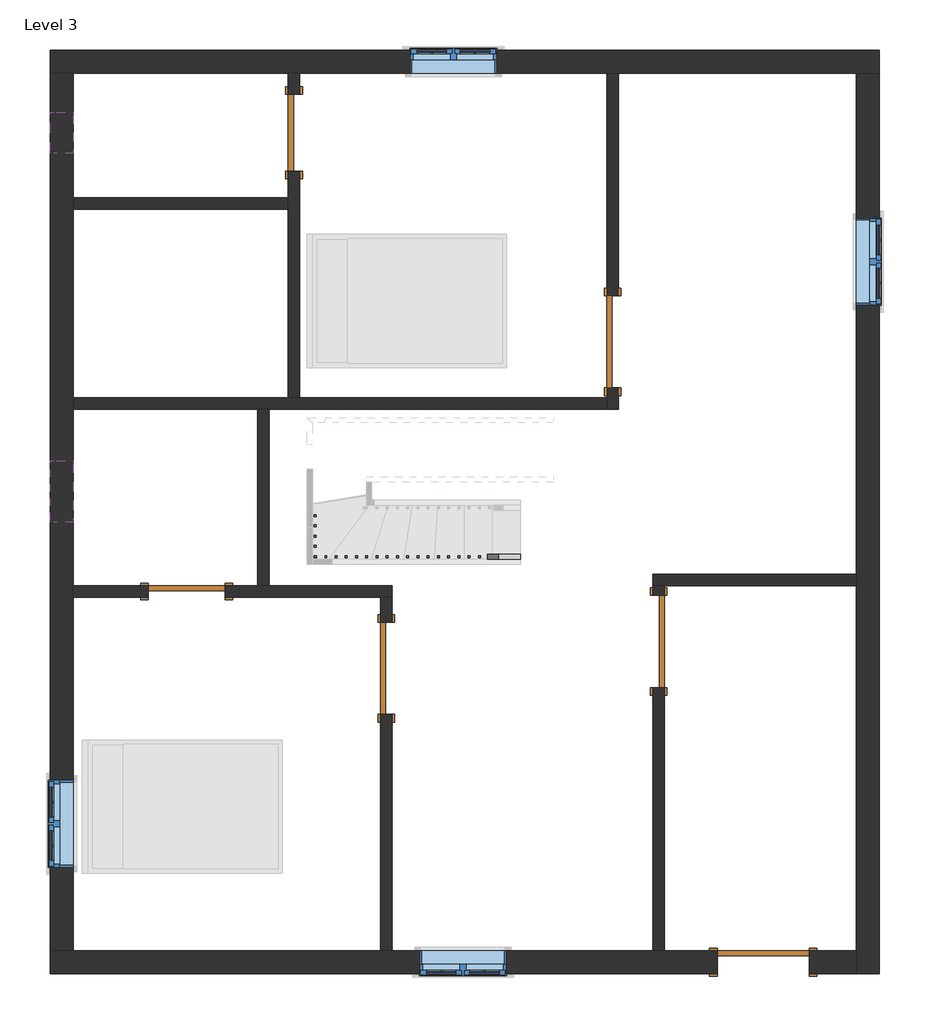
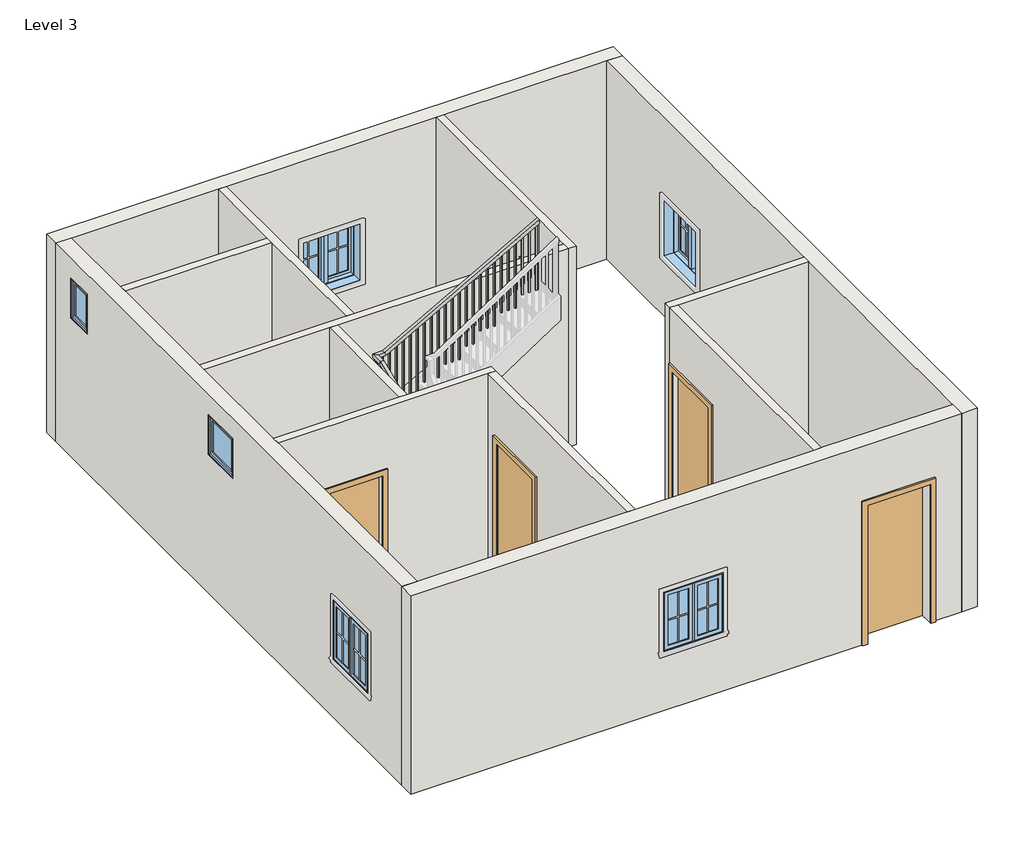
# One storey, part 1 of 2: 13 walls, 6 doors, 6 windows, 1 railing.
"""IFC4 building model written with IfcOpenShell, lengths in millimetres."""

from ifc_helpers import new_model, si_unit, frame, origin, place, context, project, spatial, polyline, outline, extrude, faceted_brep, transform, mapped, element, save
from components import door_d8f5dbb5, door_f2b275c1, door_305aa2a5, door_e5f9f3c4, door_0ca8825f, window_aa618e30, window_80340324, window_339605e1

model = new_model("IFC4")

# Units and contexts
model_context = context("Model", 3, world=origin())
ifc_project = project(units=[si_unit("LENGTHUNIT", "METRE", prefix="MILLI")], contexts=[model_context])

# Site, building, storey
site = spatial("IfcSite", under=ifc_project)
building = spatial("IfcBuilding", under=site)
storey = spatial("IfcBuildingStorey", under=building, Name="Level 3", Elevation=3200.4)

# Doors
placement = place(None, origin())
door_shape = door_d8f5dbb5(model_context)
element("IfcDoor", 1, ObjectType="Single-Flush : 30\" x 80\"", at=placement, inside=storey, context=model_context, shape_type="MappedRepresentation", body=[
    mapped(door_shape, transform((-2510.1648498, 3958.5558073, 3200.4), x_axis=(0.0, 1.0, 0.0), y_axis=(-1.0, 0.0, 0.0), z_axis=(0.0, 0.0, 1.0))),
])
door_2_shape = door_f2b275c1(model_context)
element("IfcDoor", 2, ObjectType="Single-Flush : 30\" x 80\"", at=placement, inside=storey, context=model_context, shape_type="MappedRepresentation", body=[
    mapped(door_2_shape, transform((-3576.9648498, -592.8066927, 3200.4), x_axis=(-1.0, 0.0, 0.0), y_axis=(0.0, -1.0, 0.0), z_axis=(0.0, 0.0, 1.0))),
])
door_3_shape = door_305aa2a5(model_context)
element("IfcDoor", 3, ObjectType="Single-Flush : 36\" x 84\"", at=placement, inside=storey, context=model_context, shape_type="MappedRepresentation", body=[
    mapped(door_3_shape, transform((652.1351502, 1883.6933073, 3200.4), x_axis=(0.0, -1.0, 0.0), y_axis=(1.0, 0.0, 0.0), z_axis=(0.0, 0.0, 1.0))),
])
element("IfcDoor", 4, ObjectType="Single-Flush : 36\" x 84\"", at=placement, inside=storey, context=model_context, shape_type="MappedRepresentation", body=[
    mapped(door_3_shape, transform((1109.3351502, -1088.1066927, 3200.4), x_axis=(0.0, 1.0, 0.0), y_axis=(-1.0, 0.0, 0.0), z_axis=(0.0, 0.0, 1.0))),
])
door_4_shape = door_e5f9f3c4(model_context)
element("IfcDoor", 5, ObjectType="Single-Flush : 36\" x 84\"", at=placement, inside=storey, context=model_context, shape_type="MappedRepresentation", body=[
    mapped(door_4_shape, transform((-1595.7648498, -1354.8066927, 3200.4), x_axis=(0.0, 1.0, 0.0), y_axis=(-1.0, 0.0, 0.0), z_axis=(0.0, 0.0, 1.0))),
])
door_5_shape = door_0ca8825f(model_context)
element("IfcDoor", 6, ObjectType="Single-Flush : 36\" x 84\"", at=placement, inside=storey, context=model_context, shape_type="MappedRepresentation", body=[
    mapped(door_5_shape, transform((2147.5601502, -4269.4566927, 3200.4), x_axis=(1.0, 0.0, 0.0), y_axis=(0.0, 1.0, 0.0), z_axis=(0.0, 0.0, 1.0))),
])

# Railing
element("IfcRailing", 7, ObjectType="Handrail - Rectangular", at=placement, inside=storey, context=model_context, shape_type="SolidModel", body=[
    faceted_brep([(-264.8831579, -271.8029286, 4284.1333333), (-264.8831579, -271.8029286, 4226.5518622), (-264.8831579, -221.0029286, 4226.5518622), (-264.8831579, -221.0029286, 4284.1333333), (-2203.3957557, -271.8029286, 5318.666441), (-2216.1029055, -271.8029286, 5267.866441), (-2216.1029055, -221.0029286, 5267.866441), (-2203.3957557, -221.0029286, 5318.666441), (-2328.8610857, -271.8029286, 5318.666441), (-2328.8610857, -271.8029286, 5267.866441), (-2278.0610857, -221.0029286, 5267.866441), (-2278.0610857, -221.0029286, 5318.666441), (-2328.8610857, -117.3180853, 5318.666441), (-2328.8610857, -107.2249429, 5267.866441), (-2278.0610857, -107.2249429, 5267.866441), (-2278.0610857, -117.3180853, 5318.666441), (-2328.8610857, 889.2076495, 5735.0648193), (-2328.8610857, 899.300792, 5684.2648193), (-2278.0610857, 899.300792, 5684.2648193), (-2278.0610857, 889.2076495, 5735.0648193), (-2328.8610857, 1080.0895433, 5735.0648193), (-2328.8610857, 1080.0895433, 5684.2648193), (-2278.0610857, 1029.2895433, 5684.2648193), (-2278.0610857, 1029.2895433, 5735.0648193), (-2181.3423106, 1080.0895433, 5735.0648193), (-2168.0744201, 1080.0895433, 5684.2648193), (-2168.0744201, 1029.2895433, 5684.2648193), (-2181.3423106, 1029.2895433, 5735.0648193), (63.4034409, 1080.0895433, 6993.4666667), (63.4034409, 1029.2895433, 6993.4666667), (63.4034409, 1029.2895433, 6935.2287027), (63.4034409, 1080.0895433, 6935.2287027)], [[[0, 1, 2, 3]], [[1, 0, 4, 5]], [[2, 1, 5, 6]], [[3, 2, 6, 7]], [[0, 3, 7, 4]], [[5, 4, 8, 9]], [[6, 5, 9, 10]], [[7, 6, 10, 11]], [[4, 7, 11, 8]], [[9, 8, 12, 13]], [[10, 9, 13, 14]], [[11, 10, 14, 15]], [[8, 11, 15, 12]], [[13, 12, 16, 17]], [[14, 13, 17, 18]], [[15, 14, 18, 19]], [[12, 15, 19, 16]], [[17, 16, 20, 21]], [[18, 17, 21, 22]], [[19, 18, 22, 23]], [[16, 19, 23, 20]], [[21, 20, 24, 25]], [[22, 21, 25, 26]], [[23, 22, 26, 27]], [[20, 23, 27, 24]], [[28, 29, 30, 31]], [[25, 24, 28, 31]], [[26, 25, 31, 30]], [[27, 26, 30, 29]], [[24, 27, 29, 28]]]),
    extrude(outline(polyline([(6913.0348603, 23.8139143), (5909.7333333, 23.8139143), (5909.7333333, 42.8639143), (6923.7142681, 42.8639143), (6913.0348603, 23.8139143)])), frame((0.0, 1045.1645433, 0.0), z_axis=(0.0, 1.0, 0.0), x_axis=(0.0, 0.0, 1.0)), (0.0, 0.0, 1.0), 19.05),
    extrude(outline(polyline([(6856.078019, -77.7860857), (5909.7333333, -77.7860857), (5909.7333333, -58.7360857), (6866.7574267, -58.7360857), (6856.078019, -77.7860857)])), frame((0.0, 1045.1645433, 0.0), z_axis=(0.0, 1.0, 0.0), x_axis=(0.0, 0.0, 1.0)), (0.0, 0.0, 1.0), 19.05),
    extrude(outline(polyline([(6799.1211776, -179.3860857), (5909.7333333, -179.3860857), (5909.7333333, -160.3360857), (6809.8005853, -160.3360857), (6799.1211776, -179.3860857)])), frame((0.0, 1045.1645433, 0.0), z_axis=(0.0, 1.0, 0.0), x_axis=(0.0, 0.0, 1.0)), (0.0, 0.0, 1.0), 19.05),
    extrude(outline(polyline([(6742.1643362, -280.9860857), (5740.4, -280.9860857), (5740.4, -261.9360857), (6752.843744, -261.9360857), (6742.1643362, -280.9860857)])), frame((0.0, 1045.1645433, 0.0), z_axis=(0.0, 1.0, 0.0), x_axis=(0.0, 0.0, 1.0)), (0.0, 0.0, 1.0), 19.05),
    extrude(outline(polyline([(6685.2074948, -382.5860857), (5740.4, -382.5860857), (5740.4, -363.5360857), (6695.8869026, -363.5360857), (6685.2074948, -382.5860857)])), frame((0.0, 1045.1645433, 0.0), z_axis=(0.0, 1.0, 0.0), x_axis=(0.0, 0.0, 1.0)), (0.0, 0.0, 1.0), 19.05),
    extrude(outline(polyline([(6628.2506535, -484.1860857), (5740.4, -484.1860857), (5740.4, -465.1360857), (6638.9300612, -465.1360857), (6628.2506535, -484.1860857)])), frame((0.0, 1045.1645433, 0.0), z_axis=(0.0, 1.0, 0.0), x_axis=(0.0, 0.0, 1.0)), (0.0, 0.0, 1.0), 19.05),
    extrude(outline(polyline([(6571.2938121, -585.7860857), (5571.0666667, -585.7860857), (5571.0666667, -566.7360857), (6581.9732198, -566.7360857), (6571.2938121, -585.7860857)])), frame((0.0, 1045.1645433, 0.0), z_axis=(0.0, 1.0, 0.0), x_axis=(0.0, 0.0, 1.0)), (0.0, 0.0, 1.0), 19.05),
    extrude(outline(polyline([(6514.3369707, -687.3860857), (5571.0666667, -687.3860857), (5571.0666667, -668.3360857), (6525.0163785, -668.3360857), (6514.3369707, -687.3860857)])), frame((0.0, 1045.1645433, 0.0), z_axis=(0.0, 1.0, 0.0), x_axis=(0.0, 0.0, 1.0)), (0.0, 0.0, 1.0), 19.05),
    extrude(outline(polyline([(6457.3801293, -788.9860857), (5571.0666667, -788.9860857), (5571.0666667, -769.9360857), (6468.0595371, -769.9360857), (6457.3801293, -788.9860857)])), frame((0.0, 1045.1645433, 0.0), z_axis=(0.0, 1.0, 0.0), x_axis=(0.0, 0.0, 1.0)), (0.0, 0.0, 1.0), 19.05),
    extrude(outline(polyline([(6400.423288, -890.5860857), (5401.7333333, -890.5860857), (5401.7333333, -871.5360857), (6411.1026957, -871.5360857), (6400.423288, -890.5860857)])), frame((0.0, 1045.1645433, 0.0), z_axis=(0.0, 1.0, 0.0), x_axis=(0.0, 0.0, 1.0)), (0.0, 0.0, 1.0), 19.05),
    extrude(outline(polyline([(6343.4664466, -992.1860857), (5401.7333333, -992.1860857), (5401.7333333, -973.1360857), (6354.1458543, -973.1360857), (6343.4664466, -992.1860857)])), frame((0.0, 1045.1645433, 0.0), z_axis=(0.0, 1.0, 0.0), x_axis=(0.0, 0.0, 1.0)), (0.0, 0.0, 1.0), 19.05),
    extrude(outline(polyline([(6286.5096052, -1093.7860857), (5232.4, -1093.7860857), (5232.4, -1074.7360857), (6297.189013, -1074.7360857), (6286.5096052, -1093.7860857)])), frame((0.0, 1045.1645433, 0.0), z_axis=(0.0, 1.0, 0.0), x_axis=(0.0, 0.0, 1.0)), (0.0, 0.0, 1.0), 19.05),
    extrude(outline(polyline([(6229.5527638, -1195.3860857), (5232.4, -1195.3860857), (5232.4, -1176.3360857), (6240.2321716, -1176.3360857), (6229.5527638, -1195.3860857)])), frame((0.0, 1045.1645433, 0.0), z_axis=(0.0, 1.0, 0.0), x_axis=(0.0, 0.0, 1.0)), (0.0, 0.0, 1.0), 19.05),
    extrude(outline(polyline([(6172.5959225, -1296.9860857), (5232.4, -1296.9860857), (5232.4, -1277.9360857), (6183.2753302, -1277.9360857), (6172.5959225, -1296.9860857)])), frame((0.0, 1045.1645433, 0.0), z_axis=(0.0, 1.0, 0.0), x_axis=(0.0, 0.0, 1.0)), (0.0, 0.0, 1.0), 19.05),
    extrude(outline(polyline([(6115.6390811, -1398.5860857), (5063.0666667, -1398.5860857), (5063.0666667, -1379.5360857), (6126.3184889, -1379.5360857), (6115.6390811, -1398.5860857)])), frame((0.0, 1045.1645433, 0.0), z_axis=(0.0, 1.0, 0.0), x_axis=(0.0, 0.0, 1.0)), (0.0, 0.0, 1.0), 19.05),
    extrude(outline(polyline([(6058.6822397, -1500.1860857), (5063.0666667, -1500.1860857), (5063.0666667, -1481.1360857), (6069.3616475, -1481.1360857), (6058.6822397, -1500.1860857)])), frame((0.0, 1045.1645433, 0.0), z_axis=(0.0, 1.0, 0.0), x_axis=(0.0, 0.0, 1.0)), (0.0, 0.0, 1.0), 19.05),
    extrude(outline(polyline([(6001.7253983, -1601.7860857), (5063.0666667, -1601.7860857), (5063.0666667, -1582.7360857), (6012.4048061, -1582.7360857), (6001.7253983, -1601.7860857)])), frame((0.0, 1045.1645433, 0.0), z_axis=(0.0, 1.0, 0.0), x_axis=(0.0, 0.0, 1.0)), (0.0, 0.0, 1.0), 19.05),
    extrude(outline(polyline([(5944.768557, -1703.3860857), (4893.7333333, -1703.3860857), (4893.7333333, -1684.3360857), (5955.4479647, -1684.3360857), (5944.768557, -1703.3860857)])), frame((0.0, 1045.1645433, 0.0), z_axis=(0.0, 1.0, 0.0), x_axis=(0.0, 0.0, 1.0)), (0.0, 0.0, 1.0), 19.05),
    extrude(outline(polyline([(5887.8117156, -1804.9860857), (4893.7333333, -1804.9860857), (4893.7333333, -1785.9360857), (5898.4911234, -1785.9360857), (5887.8117156, -1804.9860857)])), frame((0.0, 1045.1645433, 0.0), z_axis=(0.0, 1.0, 0.0), x_axis=(0.0, 0.0, 1.0)), (0.0, 0.0, 1.0), 19.05),
    extrude(outline(polyline([(5830.8548742, -1906.5860857), (4893.7333333, -1906.5860857), (4893.7333333, -1887.5360857), (5841.534282, -1887.5360857), (5830.8548742, -1906.5860857)])), frame((0.0, 1045.1645433, 0.0), z_axis=(0.0, 1.0, 0.0), x_axis=(0.0, 0.0, 1.0)), (0.0, 0.0, 1.0), 19.05),
    extrude(outline(polyline([(5773.8980329, -2008.1860857), (4893.7333333, -2008.1860857), (4893.7333333, -1989.1360857), (5784.5774406, -1989.1360857), (5773.8980329, -2008.1860857)])), frame((0.0, 1045.1645433, 0.0), z_axis=(0.0, 1.0, 0.0), x_axis=(0.0, 0.0, 1.0)), (0.0, 0.0, 1.0), 19.05),
    extrude(outline(polyline([(5716.9411915, -2109.7860857), (4724.4, -2109.7860857), (4724.4, -2090.7360857), (5727.6205992, -2090.7360857), (5716.9411915, -2109.7860857)])), frame((0.0, 1045.1645433, 0.0), z_axis=(0.0, 1.0, 0.0), x_axis=(0.0, 0.0, 1.0)), (0.0, 0.0, 1.0), 19.05),
    extrude(outline(polyline([(-2211.3860857, 1064.2145433), (-2192.3360857, 1064.2145433), (-2192.3360857, 1045.1645433), (-2211.3860857, 1045.1645433), (-2211.3860857, 1064.2145433)])), frame((0.0, 0.0, 4724.4), z_axis=(0.0, 0.0, 1.0), x_axis=(1.0, 0.0, 0.0)), (0.0, 0.0, 1.0), 959.8648193),
    extrude(outline(polyline([(-2312.9860857, 963.2720714), (-2312.9860857, 982.3220714), (-2293.9360857, 982.3220714), (-2293.9360857, 963.2720714), (-2312.9860857, 963.2720714)])), frame((0.0, 0.0, 4724.4), z_axis=(0.0, 0.0, 1.0), x_axis=(1.0, 0.0, 0.0)), (0.0, 0.0, 1.0), 959.8648193),
    extrude(outline(polyline([(880.7220714, 5676.5788269), (880.7220714, 4724.4), (861.6720714, 4724.4), (861.6720714, 5668.6978669), (880.7220714, 5676.5788269)])), frame((-2312.9860857, 0.0, 0.0), z_axis=(1.0, 0.0, 0.0), x_axis=(0.0, 1.0, 0.0)), (0.0, 0.0, 1.0), 19.05),
    extrude(outline(polyline([(779.1220714, 5634.54704), (779.1220714, 4724.4), (760.0720714, 4724.4), (760.0720714, 5626.6660799), (779.1220714, 5634.54704)])), frame((-2312.9860857, 0.0, 0.0), z_axis=(1.0, 0.0, 0.0), x_axis=(0.0, 1.0, 0.0)), (0.0, 0.0, 1.0), 19.05),
    extrude(outline(polyline([(677.5220714, 5592.515253), (677.5220714, 4724.4), (658.4720714, 4724.4), (658.4720714, 5584.634293), (677.5220714, 5592.515253)])), frame((-2312.9860857, 0.0, 0.0), z_axis=(1.0, 0.0, 0.0), x_axis=(0.0, 1.0, 0.0)), (0.0, 0.0, 1.0), 19.05),
    extrude(outline(polyline([(575.9220714, 5550.4834661), (575.9220714, 4555.0666667), (556.8720714, 4555.0666667), (556.8720714, 5542.602506), (575.9220714, 5550.4834661)])), frame((-2312.9860857, 0.0, 0.0), z_axis=(1.0, 0.0, 0.0), x_axis=(0.0, 1.0, 0.0)), (0.0, 0.0, 1.0), 19.05),
    extrude(outline(polyline([(474.3220714, 5508.4516792), (474.3220714, 4555.0666667), (455.2720714, 4555.0666667), (455.2720714, 5500.5707191), (474.3220714, 5508.4516792)])), frame((-2312.9860857, 0.0, 0.0), z_axis=(1.0, 0.0, 0.0), x_axis=(0.0, 1.0, 0.0)), (0.0, 0.0, 1.0), 19.05),
    extrude(outline(polyline([(372.7220714, 5466.4198922), (372.7220714, 4555.0666667), (353.6720714, 4555.0666667), (353.6720714, 5458.5389322), (372.7220714, 5466.4198922)])), frame((-2312.9860857, 0.0, 0.0), z_axis=(1.0, 0.0, 0.0), x_axis=(0.0, 1.0, 0.0)), (0.0, 0.0, 1.0), 19.05),
    extrude(outline(polyline([(271.1220714, 5424.3881053), (271.1220714, 4555.0666667), (252.0720714, 4555.0666667), (252.0720714, 5416.5071452), (271.1220714, 5424.3881053)])), frame((-2312.9860857, 0.0, 0.0), z_axis=(1.0, 0.0, 0.0), x_axis=(0.0, 1.0, 0.0)), (0.0, 0.0, 1.0), 19.05),
    extrude(outline(polyline([(169.5220714, 5382.3563183), (169.5220714, 4385.7333333), (150.4720714, 4385.7333333), (150.4720714, 5374.4753583), (169.5220714, 5382.3563183)])), frame((-2312.9860857, 0.0, 0.0), z_axis=(1.0, 0.0, 0.0), x_axis=(0.0, 1.0, 0.0)), (0.0, 0.0, 1.0), 19.05),
    extrude(outline(polyline([(67.9220714, 5340.3245314), (67.9220714, 4385.7333333), (48.8720714, 4385.7333333), (48.8720714, 5332.4435714), (67.9220714, 5340.3245314)])), frame((-2312.9860857, 0.0, 0.0), z_axis=(1.0, 0.0, 0.0), x_axis=(0.0, 1.0, 0.0)), (0.0, 0.0, 1.0), 19.05),
    extrude(outline(polyline([(-33.6779286, 5298.2927445), (-33.6779286, 4385.7333333), (-52.7279286, 4385.7333333), (-52.7279286, 5290.4117844), (-33.6779286, 5298.2927445)])), frame((-2312.9860857, 0.0, 0.0), z_axis=(1.0, 0.0, 0.0), x_axis=(0.0, 1.0, 0.0)), (0.0, 0.0, 1.0), 19.05),
    extrude(outline(polyline([(-2312.9860857, -154.3279286), (-2312.9860857, -135.2779286), (-2293.9360857, -135.2779286), (-2293.9360857, -154.3279286), (-2312.9860857, -154.3279286)])), frame((0.0, 0.0, 4385.7333333), z_axis=(0.0, 0.0, 1.0), x_axis=(1.0, 0.0, 0.0)), (0.0, 0.0, 1.0), 882.1331077),
    extrude(outline(polyline([(-2287.3581579, -255.9279286), (-2306.4081579, -255.9279286), (-2306.4081579, -236.8779286), (-2287.3581579, -236.8779286), (-2287.3581579, -255.9279286)])), frame((0.0, 0.0, 4385.7333333), z_axis=(0.0, 0.0, 1.0), x_axis=(1.0, 0.0, 0.0)), (0.0, 0.0, 1.0), 882.1331077),
    extrude(outline(polyline([(5261.8387317, -2204.8081579), (4385.7333333, -2204.8081579), (4385.7333333, -2185.7581579), (5251.6722486, -2185.7581579), (5261.8387317, -2204.8081579)])), frame((0.0, -255.9279286, 0.0), z_axis=(0.0, 1.0, 0.0), x_axis=(0.0, 0.0, 1.0)), (0.0, 0.0, 1.0), 19.05),
    extrude(outline(polyline([(5207.6174882, -2103.2081579), (4216.4, -2103.2081579), (4216.4, -2084.1581579), (5197.451005, -2084.1581579), (5207.6174882, -2103.2081579)])), frame((0.0, -255.9279286, 0.0), z_axis=(0.0, 1.0, 0.0), x_axis=(0.0, 0.0, 1.0)), (0.0, 0.0, 1.0), 19.05),
    extrude(outline(polyline([(5153.3962446, -2001.6081579), (4216.4, -2001.6081579), (4216.4, -1982.5581579), (5143.2297614, -1982.5581579), (5153.3962446, -2001.6081579)])), frame((0.0, -255.9279286, 0.0), z_axis=(0.0, 1.0, 0.0), x_axis=(0.0, 0.0, 1.0)), (0.0, 0.0, 1.0), 19.05),
    extrude(outline(polyline([(5099.175001, -1900.0081579), (4216.4, -1900.0081579), (4216.4, -1880.9581579), (5089.0085178, -1880.9581579), (5099.175001, -1900.0081579)])), frame((0.0, -255.9279286, 0.0), z_axis=(0.0, 1.0, 0.0), x_axis=(0.0, 0.0, 1.0)), (0.0, 0.0, 1.0), 19.05),
    extrude(outline(polyline([(5044.9537574, -1798.4081579), (4216.4, -1798.4081579), (4216.4, -1779.3581579), (5034.7872743, -1779.3581579), (5044.9537574, -1798.4081579)])), frame((0.0, -255.9279286, 0.0), z_axis=(0.0, 1.0, 0.0), x_axis=(0.0, 0.0, 1.0)), (0.0, 0.0, 1.0), 19.05),
    extrude(outline(polyline([(4990.7325139, -1696.8081579), (4047.0666667, -1696.8081579), (4047.0666667, -1677.7581579), (4980.5660307, -1677.7581579), (4990.7325139, -1696.8081579)])), frame((0.0, -255.9279286, 0.0), z_axis=(0.0, 1.0, 0.0), x_axis=(0.0, 0.0, 1.0)), (0.0, 0.0, 1.0), 19.05),
    extrude(outline(polyline([(4936.5112703, -1595.2081579), (4047.0666667, -1595.2081579), (4047.0666667, -1576.1581579), (4926.3447871, -1576.1581579), (4936.5112703, -1595.2081579)])), frame((0.0, -255.9279286, 0.0), z_axis=(0.0, 1.0, 0.0), x_axis=(0.0, 0.0, 1.0)), (0.0, 0.0, 1.0), 19.05),
    extrude(outline(polyline([(4882.2900267, -1493.6081579), (4047.0666667, -1493.6081579), (4047.0666667, -1474.5581579), (4872.1235435, -1474.5581579), (4882.2900267, -1493.6081579)])), frame((0.0, -255.9279286, 0.0), z_axis=(0.0, 1.0, 0.0), x_axis=(0.0, 0.0, 1.0)), (0.0, 0.0, 1.0), 19.05),
    extrude(outline(polyline([(4828.0687831, -1392.0081579), (3877.7333333, -1392.0081579), (3877.7333333, -1372.9581579), (4817.9023, -1372.9581579), (4828.0687831, -1392.0081579)])), frame((0.0, -255.9279286, 0.0), z_axis=(0.0, 1.0, 0.0), x_axis=(0.0, 0.0, 1.0)), (0.0, 0.0, 1.0), 19.05),
    extrude(outline(polyline([(4773.8475396, -1290.4081579), (3877.7333333, -1290.4081579), (3877.7333333, -1271.3581579), (4763.6810564, -1271.3581579), (4773.8475396, -1290.4081579)])), frame((0.0, -255.9279286, 0.0), z_axis=(0.0, 1.0, 0.0), x_axis=(0.0, 0.0, 1.0)), (0.0, 0.0, 1.0), 19.05),
    extrude(outline(polyline([(4719.626296, -1188.8081579), (3877.7333333, -1188.8081579), (3877.7333333, -1169.7581579), (4709.4598128, -1169.7581579), (4719.626296, -1188.8081579)])), frame((0.0, -255.9279286, 0.0), z_axis=(0.0, 1.0, 0.0), x_axis=(0.0, 0.0, 1.0)), (0.0, 0.0, 1.0), 19.05),
    extrude(outline(polyline([(4665.4050524, -1087.2081579), (3708.4, -1087.2081579), (3708.4, -1068.1581579), (4655.2385692, -1068.1581579), (4665.4050524, -1087.2081579)])), frame((0.0, -255.9279286, 0.0), z_axis=(0.0, 1.0, 0.0), x_axis=(0.0, 0.0, 1.0)), (0.0, 0.0, 1.0), 19.05),
    extrude(outline(polyline([(4611.1838088, -985.6081579), (3708.4, -985.6081579), (3708.4, -966.5581579), (4601.0173257, -966.5581579), (4611.1838088, -985.6081579)])), frame((0.0, -255.9279286, 0.0), z_axis=(0.0, 1.0, 0.0), x_axis=(0.0, 0.0, 1.0)), (0.0, 0.0, 1.0), 19.05),
    extrude(outline(polyline([(4556.9625653, -884.0081579), (3708.4, -884.0081579), (3708.4, -864.9581579), (4546.7960821, -864.9581579), (4556.9625653, -884.0081579)])), frame((0.0, -255.9279286, 0.0), z_axis=(0.0, 1.0, 0.0), x_axis=(0.0, 0.0, 1.0)), (0.0, 0.0, 1.0), 19.05),
    extrude(outline(polyline([(4502.7413217, -782.4081579), (3539.0666667, -782.4081579), (3539.0666667, -763.3581579), (4492.5748385, -763.3581579), (4502.7413217, -782.4081579)])), frame((0.0, -255.9279286, 0.0), z_axis=(0.0, 1.0, 0.0), x_axis=(0.0, 0.0, 1.0)), (0.0, 0.0, 1.0), 19.05),
    extrude(outline(polyline([(4448.5200781, -680.8081579), (3539.0666667, -680.8081579), (3539.0666667, -661.7581579), (4438.3535949, -661.7581579), (4448.5200781, -680.8081579)])), frame((0.0, -255.9279286, 0.0), z_axis=(0.0, 1.0, 0.0), x_axis=(0.0, 0.0, 1.0)), (0.0, 0.0, 1.0), 19.05),
    extrude(outline(polyline([(4394.2988345, -579.2081579), (3539.0666667, -579.2081579), (3539.0666667, -560.1581579), (4384.1323514, -560.1581579), (4394.2988345, -579.2081579)])), frame((0.0, -255.9279286, 0.0), z_axis=(0.0, 1.0, 0.0), x_axis=(0.0, 0.0, 1.0)), (0.0, 0.0, 1.0), 19.05),
    extrude(outline(polyline([(4340.077591, -477.6081579), (3369.7333333, -477.6081579), (3369.7333333, -458.5581579), (4329.9111078, -458.5581579), (4340.077591, -477.6081579)])), frame((0.0, -255.9279286, 0.0), z_axis=(0.0, 1.0, 0.0), x_axis=(0.0, 0.0, 1.0)), (0.0, 0.0, 1.0), 19.05),
    extrude(outline(polyline([(4285.8563474, -376.0081579), (3369.7333333, -376.0081579), (3369.7333333, -356.9581579), (4275.6898642, -356.9581579), (4285.8563474, -376.0081579)])), frame((0.0, -255.9279286, 0.0), z_axis=(0.0, 1.0, 0.0), x_axis=(0.0, 0.0, 1.0)), (0.0, 0.0, 1.0), 19.05),
    extrude(outline(polyline([(-2312.9860857, 1045.1645433), (-2312.9860857, 1064.2145433), (-2293.9360857, 1064.2145433), (-2293.9360857, 1045.1645433), (-2312.9860857, 1045.1645433)])), frame((0.0, 0.0, 4724.4), z_axis=(0.0, 0.0, 1.0), x_axis=(1.0, 0.0, 0.0)), (0.0, 0.0, 1.0), 959.8648193),
    extrude(outline(polyline([(-2293.9360857, -255.9279286), (-2312.9860857, -255.9279286), (-2312.9860857, -236.8779286), (-2293.9360857, -236.8779286), (-2293.9360857, -255.9279286)])), frame((0.0, 0.0, 4385.7333333), z_axis=(0.0, 0.0, 1.0), x_axis=(1.0, 0.0, 0.0)), (0.0, 0.0, 1.0), 882.1331077),
    extrude(outline(polyline([(6924.549295, 44.3534409), (5909.7333333, 44.3534409), (5909.7333333, 63.4034409), (6935.2287027, 63.4034409), (6924.549295, 44.3534409)])), frame((0.0, 1045.1645433, 0.0), z_axis=(0.0, 1.0, 0.0), x_axis=(0.0, 0.0, 1.0)), (0.0, 0.0, 1.0), 19.05),
    extrude(outline(polyline([(4236.7183454, -283.9331579), (3369.7333333, -283.9331579), (3369.7333333, -264.8831579), (4226.5518622, -264.8831579), (4236.7183454, -283.9331579)])), frame((0.0, -255.9279286, 0.0), z_axis=(0.0, 1.0, 0.0), x_axis=(0.0, 0.0, 1.0)), (0.0, 0.0, 1.0), 19.05),
])

# Walls
element("IfcWall", 8, ObjectType="WALL4.5\"", at=placement, inside=storey, context=model_context, shape_type="SweptSolid", body=[
    extrude(outline(polyline([(-2567.3148498, 3198.1433073), (-4700.9148498, 3198.1433073), (-4700.9148498, 3312.4433073), (-2567.3148498, 3312.4433073), (-2567.3148498, 3198.1433073)])), frame((0.0, 0.0, 3200.4), z_axis=(0.0, 0.0, 1.0), x_axis=(1.0, 0.0, 0.0)), (0.0, 0.0, 1.0), 3048.0),
])
element("IfcWall", 9, ObjectType="WALL4.5\"", at=placement, inside=storey, context=model_context, shape_type="Brep", body=[
    faceted_brep([(-2567.3148498, 4547.5183073, 3200.4), (-2567.3148498, 4339.5558073, 3200.4), (-2567.3148498, 4339.5558073, 5232.4), (-2567.3148498, 3577.5558073, 5232.4), (-2567.3148498, 3577.5558073, 3200.4), (-2567.3148498, 3312.4433073, 3200.4), (-2567.3148498, 3198.1433073, 3200.4), (-2567.3148498, 1331.2433073, 3200.4), (-2567.3148498, 1331.2433073, 6248.4), (-2567.3148498, 3198.1433073, 6248.4), (-2567.3148498, 3312.4433073, 6248.4), (-2567.3148498, 4547.5183073, 6248.4), (-2453.0148498, 4339.5558073, 5232.4), (-2453.0148498, 4339.5558073, 3200.4), (-2453.0148498, 4547.5183073, 3200.4), (-2453.0148498, 4547.5183073, 6248.4), (-2453.0148498, 1331.2433073, 6248.4), (-2453.0148498, 1331.2433073, 3200.4), (-2453.0148498, 3577.5558073, 3200.4), (-2453.0148498, 3577.5558073, 5232.4)], [[[0, 1, 2, 3, 4, 5, 6, 7, 8, 9, 10, 11]], [[12, 13, 14, 15, 16, 17, 18, 19]], [[18, 17, 7, 6, 5, 4]], [[14, 13, 1, 0]], [[0, 11, 15, 14]], [[8, 7, 17, 16]], [[2, 1, 13, 12]], [[3, 2, 12, 19]], [[4, 3, 19, 18]], [[11, 10, 9, 8, 16, 15]]]),
])
element("IfcWall", 10, ObjectType="WALL4.5\"", at=placement, inside=storey, context=model_context, shape_type="Brep", body=[
    faceted_brep([(594.9851502, 1426.4933073, 5334.0), (594.9851502, 1426.4933073, 3200.4), (594.9851502, 1331.2433073, 3200.4), (594.9851502, 1216.9433073, 3200.4), (594.9851502, 1216.9433073, 6248.4), (594.9851502, 1331.2433073, 6248.4), (594.9851502, 4547.5183073, 6248.4), (594.9851502, 4547.5183073, 3200.4), (594.9851502, 2340.8933073, 3200.4), (594.9851502, 2340.8933073, 5334.0), (709.2851502, 1216.9433073, 3200.4), (709.2851502, 1426.4933073, 3200.4), (709.2851502, 1426.4933073, 5334.0), (709.2851502, 2340.8933073, 5334.0), (709.2851502, 2340.8933073, 3200.4), (709.2851502, 4547.5183073, 3200.4), (709.2851502, 4547.5183073, 6248.4), (709.2851502, 1216.9433073, 6248.4)], [[[0, 1, 2, 3, 4, 5, 6, 7, 8, 9]], [[10, 11, 12, 13, 14, 15, 16, 17]], [[8, 7, 15, 14]], [[3, 2, 1, 11, 10]], [[7, 6, 16, 15]], [[4, 3, 10, 17]], [[12, 11, 1, 0]], [[13, 12, 0, 9]], [[14, 13, 9, 8]], [[6, 5, 4, 17, 16]]]),
])
element("IfcWall", 11, ObjectType="WALL4.5\"", at=placement, inside=storey, context=model_context, shape_type="Brep", body=[
    faceted_brep([(-4700.9148498, 1216.9433073, 3200.4), (-2872.1148498, 1216.9433073, 3200.4), (-2757.8148498, 1216.9433073, 3200.4), (594.9851502, 1216.9433073, 3200.4), (594.9851502, 1216.9433073, 6248.4), (-2757.8148498, 1216.9433073, 6248.4), (-2872.1148498, 1216.9433073, 6248.4), (-4700.9148498, 1216.9433073, 6248.4), (-4700.9148498, 1331.2433073, 3200.4), (-4700.9148498, 1331.2433073, 6248.4), (-2567.3148498, 1331.2433073, 6248.4), (-2453.0148498, 1331.2433073, 6248.4), (594.9851502, 1331.2433073, 6248.4), (594.9851502, 1331.2433073, 3200.4), (-2453.0148498, 1331.2433073, 3200.4), (-2567.3148498, 1331.2433073, 3200.4)], [[[0, 1, 2, 3, 4, 5, 6, 7]], [[8, 9, 10, 11, 12, 13, 14, 15]], [[3, 2, 1, 0, 8, 15, 14, 13]], [[4, 3, 13, 12]], [[0, 7, 9, 8]], [[7, 6, 5, 4, 12, 11, 10, 9]]]),
])
element("IfcWall", 12, ObjectType="WALL4.5\"", at=placement, inside=storey, context=model_context, shape_type="SweptSolid", body=[
    extrude(outline(polyline([(-2872.1148498, -535.6566927), (-2872.1148498, 1216.9433073), (-2757.8148498, 1216.9433073), (-2757.8148498, -535.6566927), (-2872.1148498, -535.6566927)])), frame((0.0, 0.0, 3200.4), z_axis=(0.0, 0.0, 1.0), x_axis=(1.0, 0.0, 0.0)), (0.0, 0.0, 1.0), 3048.0),
])
element("IfcWall", 13, ObjectType="WALL4.5\"", at=placement, inside=storey, context=model_context, shape_type="Brep", body=[
    faceted_brep([(-4700.9148498, -649.9566927, 3200.4), (-3957.9648498, -649.9566927, 3200.4), (-3957.9648498, -649.9566927, 5232.4), (-3195.9648498, -649.9566927, 5232.4), (-3195.9648498, -649.9566927, 3200.4), (-1652.9148498, -649.9566927, 3200.4), (-1538.6148498, -649.9566927, 3200.4), (-1538.6148498, -649.9566927, 6248.4), (-1652.9148498, -649.9566927, 6248.4), (-4700.9148498, -649.9566927, 6248.4), (-3957.9648498, -535.6566927, 5232.4), (-3957.9648498, -535.6566927, 3200.4), (-4700.9148498, -535.6566927, 3200.4), (-4700.9148498, -535.6566927, 6248.4), (-2872.1148498, -535.6566927, 6248.4), (-2757.8148498, -535.6566927, 6248.4), (-1538.6148498, -535.6566927, 6248.4), (-1538.6148498, -535.6566927, 3200.4), (-2757.8148498, -535.6566927, 3200.4), (-2872.1148498, -535.6566927, 3200.4), (-3195.9648498, -535.6566927, 3200.4), (-3195.9648498, -535.6566927, 5232.4)], [[[0, 1, 2, 3, 4, 5, 6, 7, 8, 9]], [[10, 11, 12, 13, 14, 15, 16, 17, 18, 19, 20, 21]], [[12, 11, 1, 0]], [[20, 19, 18, 17, 6, 5, 4]], [[7, 6, 17, 16]], [[0, 9, 13, 12]], [[2, 1, 11, 10]], [[3, 2, 10, 21]], [[4, 3, 21, 20]], [[9, 8, 7, 16, 15, 14, 13]]]),
])
element("IfcWall", 14, ObjectType="WALL4.5\"", at=placement, inside=storey, context=model_context, shape_type="Brep", body=[
    faceted_brep([(3071.4851502, -421.3566927, 3200.4), (1052.1851502, -421.3566927, 3200.4), (1052.1851502, -421.3566927, 6248.4), (3071.4851502, -421.3566927, 6248.4), (3071.4851502, -535.6566927, 3200.4), (3071.4851502, -535.6566927, 6248.4), (1166.4851502, -535.6566927, 6248.4), (1052.1851502, -535.6566927, 6248.4), (1052.1851502, -535.6566927, 3200.4), (1166.4851502, -535.6566927, 3200.4)], [[[0, 1, 2, 3]], [[4, 5, 6, 7, 8, 9]], [[1, 0, 4, 9, 8]], [[0, 3, 5, 4]], [[2, 1, 8, 7]], [[3, 2, 7, 6, 5]]]),
])
element("IfcWall", 15, ObjectType="WALL4.5\"", at=placement, inside=storey, context=model_context, shape_type="SweptSolid", body=[
    extrude(outline(polyline([(-535.6566927, 3200.4), (-630.9066927, 3200.4), (-630.9066927, 5334.0), (-1545.3066927, 5334.0), (-1545.3066927, 3200.4), (-4155.1566927, 3200.4), (-4155.1566927, 6248.4), (-535.6566927, 6248.4), (-535.6566927, 3200.4)])), frame((1052.1851502, 0.0, 0.0), z_axis=(1.0, 0.0, 0.0), x_axis=(0.0, 1.0, 0.0)), (0.0, 0.0, 1.0), 114.3),
])
element("IfcWall", 16, ObjectType="WALL4.5\"", at=placement, inside=storey, context=model_context, shape_type="SweptSolid", body=[
    extrude(outline(polyline([(-649.9566927, 3200.4), (-897.6066927, 3200.4), (-897.6066927, 5334.0), (-1812.0066927, 5334.0), (-1812.0066927, 3200.4), (-4155.1566927, 3200.4), (-4155.1566927, 6248.4), (-649.9566927, 6248.4), (-649.9566927, 3200.4)])), frame((-1652.9148498, 0.0, 0.0), z_axis=(1.0, 0.0, 0.0), x_axis=(0.0, 1.0, 0.0)), (0.0, 0.0, 1.0), 114.3),
])
element("IfcWall", 17, ObjectType="WALL9\"", at=placement, inside=storey, context=model_context, shape_type="Brep", body=[
    faceted_brep([(-4929.5148498, 4547.5183073, 3200.4), (-4700.9148498, 4547.5183073, 3200.4), (-2567.3148498, 4547.5183073, 3200.4), (-2453.0148498, 4547.5183073, 3200.4), (594.9851502, 4547.5183073, 3200.4), (709.2851502, 4547.5183073, 3200.4), (3071.4851502, 4547.5183073, 3200.4), (3300.0851502, 4547.5183073, 3200.4), (3300.0851502, 4547.5183073, 6248.4), (3071.4851502, 4547.5183073, 6248.4), (709.2851502, 4547.5183073, 6248.4), (594.9851502, 4547.5183073, 6248.4), (-2453.0148498, 4547.5183073, 6248.4), (-2567.3148498, 4547.5183073, 6248.4), (-4700.9148498, 4547.5183073, 6248.4), (-4929.5148498, 4547.5183073, 6248.4), (-497.2148498, 4547.5183073, 5029.2), (-497.2148498, 4547.5183073, 4114.8), (-1360.8148498, 4547.5183073, 4114.8), (-1360.8148498, 4547.5183073, 5029.2), (-4929.5148498, 4776.1183073, 3200.4), (-4929.5148498, 4776.1183073, 6248.4), (3300.0851502, 4776.1183073, 6248.4), (3300.0851502, 4776.1183073, 3200.4), (-497.2148498, 4776.1183073, 5029.2), (-1360.8148498, 4776.1183073, 5029.2), (-1360.8148498, 4776.1183073, 4114.8), (-497.2148498, 4776.1183073, 4114.8)], [[[0, 1, 2, 3, 4, 5, 6, 7, 8, 9, 10, 11, 12, 13, 14, 15], [16, 17, 18, 19]], [[20, 21, 22, 23], [24, 25, 26, 27]], [[7, 6, 5, 4, 3, 2, 1, 0, 20, 23]], [[8, 7, 23, 22]], [[0, 15, 21, 20]], [[17, 16, 24, 27]], [[18, 17, 27, 26]], [[19, 18, 26, 25]], [[16, 19, 25, 24]], [[15, 14, 13, 12, 11, 10, 9, 8, 22, 21]]]),
])
element("IfcWall", 18, ObjectType="WALL9\"", at=placement, inside=storey, context=model_context, shape_type="Brep", body=[
    faceted_brep([(3071.4851502, 4547.5183073, 3200.4), (3071.4851502, -421.3566927, 3200.4), (3071.4851502, -535.6566927, 3200.4), (3071.4851502, -4155.1566927, 3200.4), (3071.4851502, -4383.7566927, 3200.4), (3071.4851502, -4383.7566927, 6248.4), (3071.4851502, -4155.1566927, 6248.4), (3071.4851502, -535.6566927, 6248.4), (3071.4851502, -421.3566927, 6248.4), (3071.4851502, 4547.5183073, 6248.4), (3071.4851502, 2248.8183073, 5029.2), (3071.4851502, 2248.8183073, 4114.8), (3071.4851502, 3112.4183073, 4114.8), (3071.4851502, 3112.4183073, 5029.2), (3300.0851502, 4547.5183073, 3200.4), (3300.0851502, 4547.5183073, 6248.4), (3300.0851502, -4383.7566927, 6248.4), (3300.0851502, -4383.7566927, 3200.4), (3300.0851502, 2248.8183073, 5029.2), (3300.0851502, 3112.4183073, 5029.2), (3300.0851502, 3112.4183073, 4114.8), (3300.0851502, 2248.8183073, 4114.8)], [[[0, 1, 2, 3, 4, 5, 6, 7, 8, 9], [10, 11, 12, 13]], [[14, 15, 16, 17], [18, 19, 20, 21]], [[4, 3, 2, 1, 0, 14, 17]], [[0, 9, 15, 14]], [[5, 4, 17, 16]], [[11, 10, 18, 21]], [[12, 11, 21, 20]], [[13, 12, 20, 19]], [[10, 13, 19, 18]], [[9, 8, 7, 6, 5, 16, 15]]]),
])
element("IfcWall", 19, ObjectType="WALL9\"", at=placement, inside=storey, context=model_context, shape_type="Brep", body=[
    faceted_brep([(3071.4851502, -4155.1566927, 3200.4), (2604.7601502, -4155.1566927, 3200.4), (2604.7601502, -4155.1566927, 5334.0), (1690.3601502, -4155.1566927, 5334.0), (1690.3601502, -4155.1566927, 3200.4), (1166.4851502, -4155.1566927, 3200.4), (1052.1851502, -4155.1566927, 3200.4), (-1538.6148498, -4155.1566927, 3200.4), (-1652.9148498, -4155.1566927, 3200.4), (-4700.9148498, -4155.1566927, 3200.4), (-4929.5148498, -4155.1566927, 3200.4), (-4929.5148498, -4155.1566927, 6248.4), (-4700.9148498, -4155.1566927, 6248.4), (-1652.9148498, -4155.1566927, 6248.4), (-1538.6148498, -4155.1566927, 6248.4), (1052.1851502, -4155.1566927, 6248.4), (1166.4851502, -4155.1566927, 6248.4), (3071.4851502, -4155.1566927, 6248.4), (-1265.5648498, -4155.1566927, 5029.2), (-1265.5648498, -4155.1566927, 4114.8), (-401.9648498, -4155.1566927, 4114.8), (-401.9648498, -4155.1566927, 5029.2), (2604.7601502, -4383.7566927, 5334.0), (2604.7601502, -4383.7566927, 3200.4), (3071.4851502, -4383.7566927, 3200.4), (3071.4851502, -4383.7566927, 6248.4), (-4929.5148498, -4383.7566927, 6248.4), (-4929.5148498, -4383.7566927, 3200.4), (1690.3601502, -4383.7566927, 3200.4), (1690.3601502, -4383.7566927, 5334.0), (-1265.5648498, -4383.7566927, 5029.2), (-401.9648498, -4383.7566927, 5029.2), (-401.9648498, -4383.7566927, 4114.8), (-1265.5648498, -4383.7566927, 4114.8)], [[[0, 1, 2, 3, 4, 5, 6, 7, 8, 9, 10, 11, 12, 13, 14, 15, 16, 17], [18, 19, 20, 21]], [[22, 23, 24, 25, 26, 27, 28, 29], [30, 31, 32, 33]], [[28, 27, 10, 9, 8, 7, 6, 5, 4]], [[24, 23, 1, 0]], [[0, 17, 25, 24]], [[11, 10, 27, 26]], [[19, 18, 30, 33]], [[20, 19, 33, 32]], [[21, 20, 32, 31]], [[18, 21, 31, 30]], [[17, 16, 15, 14, 13, 12, 11, 26, 25]], [[2, 1, 23, 22]], [[3, 2, 22, 29]], [[4, 3, 29, 28]]]),
])
element("IfcWall", 20, ObjectType="WALL9\"", at=placement, inside=storey, context=model_context, shape_type="Brep", body=[
    faceted_brep([(-4700.9148498, -4155.1566927, 3200.4), (-4700.9148498, -649.9566927, 3200.4), (-4700.9148498, -535.6566927, 3200.4), (-4700.9148498, 1216.9433073, 3200.4), (-4700.9148498, 1331.2433073, 3200.4), (-4700.9148498, 3198.1433073, 3200.4), (-4700.9148498, 3312.4433073, 3200.4), (-4700.9148498, 4547.5183073, 3200.4), (-4700.9148498, 4547.5183073, 6248.4), (-4700.9148498, 3312.4433073, 6248.4), (-4700.9148498, 3198.1433073, 6248.4), (-4700.9148498, 1331.2433073, 6248.4), (-4700.9148498, 1216.9433073, 6248.4), (-4700.9148498, -535.6566927, 6248.4), (-4700.9148498, -649.9566927, 6248.4), (-4700.9148498, -4155.1566927, 6248.4), (-4700.9148498, 4161.7558073, 5943.6), (-4700.9148498, 4161.7558073, 5334.0), (-4700.9148498, 3755.3558073, 5334.0), (-4700.9148498, 3755.3558073, 5943.6), (-4700.9148498, 705.7683073, 5943.6), (-4700.9148498, 705.7683073, 5334.0), (-4700.9148498, 96.1683073, 5334.0), (-4700.9148498, 96.1683073, 5943.6), (-4700.9148498, -2466.0566927, 5029.2), (-4700.9148498, -2466.0566927, 4114.8), (-4700.9148498, -3329.6566927, 4114.8), (-4700.9148498, -3329.6566927, 5029.2), (-4929.5148498, -4155.1566927, 3200.4), (-4929.5148498, -4155.1566927, 6248.4), (-4929.5148498, 4547.5183073, 6248.4), (-4929.5148498, 4547.5183073, 3200.4), (-4929.5148498, 4161.7558073, 5943.6), (-4929.5148498, 3755.3558073, 5943.6), (-4929.5148498, 3755.3558073, 5334.0), (-4929.5148498, 4161.7558073, 5334.0), (-4929.5148498, 705.7683073, 5943.6), (-4929.5148498, 96.1683073, 5943.6), (-4929.5148498, 96.1683073, 5334.0), (-4929.5148498, 705.7683073, 5334.0), (-4929.5148498, -2466.0566927, 5029.2), (-4929.5148498, -3329.6566927, 5029.2), (-4929.5148498, -3329.6566927, 4114.8), (-4929.5148498, -2466.0566927, 4114.8)], [[[0, 1, 2, 3, 4, 5, 6, 7, 8, 9, 10, 11, 12, 13, 14, 15], [16, 17, 18, 19], [20, 21, 22, 23], [24, 25, 26, 27]], [[28, 29, 30, 31], [32, 33, 34, 35], [36, 37, 38, 39], [40, 41, 42, 43]], [[7, 6, 5, 4, 3, 2, 1, 0, 28, 31]], [[8, 7, 31, 30]], [[0, 15, 29, 28]], [[17, 16, 32, 35]], [[18, 17, 35, 34]], [[19, 18, 34, 33]], [[16, 19, 33, 32]], [[21, 20, 36, 39]], [[22, 21, 39, 38]], [[23, 22, 38, 37]], [[20, 23, 37, 36]], [[25, 24, 40, 43]], [[26, 25, 43, 42]], [[27, 26, 42, 41]], [[24, 27, 41, 40]], [[15, 14, 13, 12, 11, 10, 9, 8, 30, 29]]]),
])

# Windows
window_shape = window_aa618e30(model_context)
element("IfcWindow", 21, ObjectType="Fixed : 16\" x 24\"", at=placement, inside=storey, context=model_context, shape_type="MappedRepresentation", body=[
    mapped(window_shape, transform((-4815.2148498, 3996.6558073, 4419.6), x_axis=(0.0, 1.0, 0.0), y_axis=(-1.0, 0.0, 0.0), z_axis=(0.0, 0.0, 1.0))),
])
window_2_shape = window_80340324(model_context)
element("IfcWindow", 22, ObjectType="Fixed : 24\" x 24\"", at=placement, inside=storey, context=model_context, shape_type="MappedRepresentation", body=[
    mapped(window_2_shape, transform((-4815.2148498, 439.0683073, 4419.6), x_axis=(0.0, 1.0, 0.0), y_axis=(-1.0, 0.0, 0.0), z_axis=(0.0, 0.0, 1.0))),
])
window_3_shape = window_339605e1(model_context)
element("IfcWindow", 23, ObjectType="Window-Casement-Double : 34\" x 36\"", at=placement, inside=storey, context=model_context, shape_type="MappedRepresentation", body=[
    mapped(window_3_shape, transform((-929.0148498, 4661.8183073, 3200.4), x_axis=(1.0, 0.0, 0.0), y_axis=(0.0, 1.0, 0.0), z_axis=(0.0, 0.0, 1.0))),
])
element("IfcWindow", 24, ObjectType="Window-Casement-Double : 34\" x 36\"", at=placement, inside=storey, context=model_context, shape_type="MappedRepresentation", body=[
    mapped(window_3_shape, transform((3185.7851502, 2680.6183073, 3200.4), x_axis=(0.0, -1.0, 0.0), y_axis=(1.0, 0.0, 0.0), z_axis=(0.0, 0.0, 1.0))),
])
element("IfcWindow", 25, ObjectType="Window-Casement-Double : 34\" x 36\"", at=placement, inside=storey, context=model_context, shape_type="MappedRepresentation", body=[
    mapped(window_3_shape, transform((-833.7648498, -4269.4566927, 3200.4), x_axis=(-1.0, 0.0, 0.0), y_axis=(0.0, -1.0, 0.0), z_axis=(0.0, 0.0, 1.0))),
])
element("IfcWindow", 26, ObjectType="Window-Casement-Double : 34\" x 36\"", at=placement, inside=storey, context=model_context, shape_type="MappedRepresentation", body=[
    mapped(window_3_shape, transform((-4815.2148498, -2897.8566927, 3200.4), x_axis=(0.0, 1.0, 0.0), y_axis=(-1.0, 0.0, 0.0), z_axis=(0.0, 0.0, 1.0))),
])

save(model, "model.ifc")

# Revit data of these elements
# Type "Single-Flush : 30\" x 80\""
#   Type Mark = "5"
#   Construction Type Id = "MDOOR"
#   Assembly Code = "C1020"
#   Analytic Construction = "Metal"
#   Thickness = 0' - 2"
#   Heat Transfer Coefficient (U) = 0.651978 BTU/(h·ft²·°F)
#   Height = 6' - 8"
#   Trim Projection Ext = 0' - 1"
#   Trim Projection Int = 0' - 1"
#   Trim Width = 0' - 3"
#   Width = 2' - 6"
#   Define Thermal Properties by = 1
#   Define Thermal Properties by = 1
#   Door Material = Door - Panel
#   Frame Material = Door - Frame
#   Visual Light Transmittance = 0
#   Solar Heat Gain Coefficient = 0
#   Function = (empty or 0)
#   Wall Closure = (empty or 0)
# Type "Single-Flush : 36\" x 84\""
#   Type Mark = "1"
#   Construction Type Id = "MDOOR"
#   Assembly Code = "C1020"
#   Analytic Construction = "Metal"
#   Thickness = 0' - 2"
#   Heat Transfer Coefficient (U) = 0.651978 BTU/(h·ft²·°F)
#   Height = 7' - 0"
#   Trim Projection Ext = 0' - 1"
#   Trim Projection Int = 0' - 1"
#   Trim Width = 0' - 3"
#   Width = 3' - 0"
#   Define Thermal Properties by = 1
#   Define Thermal Properties by = 1
#   Door Material = Door - Panel
#   Frame Material = Door - Frame
#   Visual Light Transmittance = 0
#   Solar Heat Gain Coefficient = 0
#   Function = (empty or 0)
#   Wall Closure = (empty or 0)
# Type "Handrail - Rectangular"
#   Assembly Code = "C2010400"
#   built-in parameter 1008612 = 0.0416667 (stored number, unit not read)
#   built-in parameter 1008611 = 0.0416667 (stored number, unit not read)
#   built-in parameter 1008609 = 0.333333 (stored number, unit not read)
#   built-in parameter 1008604 = 0.166667 (stored number, unit not read)
#   built-in parameter 1008603 = 0.166667 (stored number, unit not read)
#   Railing Height = 3' - 0"
#   built-in parameter 1008630 = 2
#   built-in parameter 1008610 = 2
#   built-in parameter 1008618 = Baluster - Square : 3/4"
# Type "WALL4.5\""
#   Assembly Code = "B2010"
#   Layers, outside or top first: 0' - 4 1/2" no material (function 1)
# Type "WALL9\""
#   Assembly Code = "B2010"
#   Layers, outside or top first: 0' - 9" no material (function 1)
# Type "Fixed : 16\" x 24\""
#   Type Mark = "4"
#   Construction Type Id = "GSP4R"
#   Assembly Code = "B2020100"
#   Analytic Construction = "1/8 in Pilkington single glazing"
#   Visual Light Transmittance = 0.9
#   Solar Heat Gain Coefficient = 0.78
#   Heat Transfer Coefficient (U) = 0.6496 BTU/(h·ft²·°F)
#   Height = 2' - 0"
#   Default Sill Height = 3' - 0"
#   Width = 1' - 4"
#   Window Inset = 0' - 0 3/4"
#   Define Thermal Properties by = 1
#   Define Thermal Properties by = 1
#   Glass Pane Material = Glass
#   Sash Material = Sash
#   Wall Closure = (empty or 0)
# Type "Fixed : 24\" x 24\""
#   Type Mark = "3"
#   Construction Type Id = "GSP4R"
#   Assembly Code = "B2020100"
#   Analytic Construction = "1/8 in Pilkington single glazing"
#   Visual Light Transmittance = 0.9
#   Solar Heat Gain Coefficient = 0.78
#   Heat Transfer Coefficient (U) = 0.6496 BTU/(h·ft²·°F)
#   Height = 2' - 0"
#   Default Sill Height = 3' - 0"
#   Width = 2' - 0"
#   Window Inset = 0' - 0 3/4"
#   Define Thermal Properties by = 1
#   Define Thermal Properties by = 1
#   Glass Pane Material = Glass
#   Sash Material = Sash
#   Wall Closure = (empty or 0)
# Type "Window-Casement-Double : 34\" x 36\""
#   Type Mark = "14"
#   Fire Rating = "0.5h"
#   Assembly Code = "B2020100"
#   Analytic Construction = "Double glazing - domestic"
#   Frame Extension [instance default] = 0' - 0 1/4"
#   Window Inset [instance default] = 0' - 0"
#   Wall Thickness [instance default] = 0' - 6"
#   Interior Wall Closure [instance default] = 0' - 2 1/4"
#   Half Width = 1' - 5"
#   Visual Light Transmittance = 0.81
#   Thermal Resistance (R) = 1.8146 (h·ft²·°F)/BTU
#   Solar Heat Gain Coefficient = 0.76
#   Rough Width = 2' - 10 1/2"
#   Rough Height = 3' - 0 1/2"
#   Height = 3' - 0"
#   Heat Transfer Coefficient (U) = 0.5511 BTU/(h·ft²·°F)
#   Exterior Wall Closure [instance default] = 0' - 1 1/4"
#   Extension Jamb [instance default] = 0' - 2 1/4"
#   Default Sill Height = 3' - 0"
#   Width = 2' - 10"
#   Define Thermal Properties by = 0
#   Muntin Visibility = yes
#   Interior Trim Visibility [instance default] = yes
#   Exterior Trim Visibility [instance default] = yes
#   Extension Jamb Visibility [instance default] = yes
#   Interior Trim Material = Wood - Stained
#   Muntin Pattern = Muntin Pattern_2x2 : Muntin Pattern_2x2
#   Interior Trim = Trim-Window-Interior-Flat : Picture Frame
#   Interior Frame Material = Wood - Stained
#   Glass Panel Material = Glass
#   Exterior Trim Material = Clad - White
#   Exterior Trim = Trim-Window-Exterior-Flat : with Sill
#   Exterior Frame Material = Clad - White
#   Wall Closure = (empty or 0)
# Elements 1, 2 (IfcDoor, "Single-Flush : 30\" x 80\"")
#   Phase Created = New Construction
#   Materials on its faces: "Door - Frame", "Door - Panel"
# Elements 3, 4, 5, 6 (IfcDoor, "Single-Flush : 36\" x 84\"")
#   Phase Created = New Construction
#   Materials on its faces: "Door - Frame", "Door - Panel"
# Element 7 (IfcRailing, "Handrail - Rectangular")
#   Phase Created = New Construction
# Elements 8, 9, 10, 11, 12, 13, 14, 15, 16 (IfcWall, "WALL4.5\"")
#   Top Offset = 0' - 0"
#   Base Offset = 0' - 0"
#   Unconnected Height = 10' - 0"
#   wall height = 10' - 0"
#   Phase Created = New Construction
#   Base Constraint = Level 3
#   Materials on its faces: "Default Wall"
# Elements 17, 18, 19, 20 (IfcWall, "WALL9\"")
#   Top Offset = 0' - 0"
#   Base Offset = 0' - 0"
#   Unconnected Height = 10' - 0"
#   wall height = 10' - 0"
#   Phase Created = New Construction
#   Base Constraint = Level 3
#   Materials on its faces: "Default Wall", "Wood - Stained"
# Element 21 (IfcWindow, "Fixed : 16\" x 24\"")
#   Mark = "10"
#   Phase Created = New Construction
#   Materials on its faces: "Sash", "Glass"
# Element 22 (IfcWindow, "Fixed : 24\" x 24\"")
#   Mark = "14"
#   Phase Created = New Construction
#   Materials on its faces: "Sash", "Glass"
# Element 23 (IfcWindow, "Window-Casement-Double : 34\" x 36\"")
#   Mark = "11"
#   Window Inset = 0' - 0"
#   Interior Wall Closure = 0' - 2 1/4"
#   Frame Extension = 0' - 0 1/4"
#   Exterior Wall Closure = 0' - 1 1/4"
#   Interior Trim Visibility = yes
#   Exterior Trim Visibility = yes
#   Phase Created = New Construction
#   Materials on its faces: "Wood - Stained", "Glass", "Clad - White"
# Element 24 (IfcWindow, "Window-Casement-Double : 34\" x 36\"")
#   Mark = "12"
#   Window Inset = 0' - 0"
#   Interior Wall Closure = 0' - 2 1/4"
#   Frame Extension = 0' - 0 1/4"
#   Exterior Wall Closure = 0' - 1 1/4"
#   Interior Trim Visibility = yes
#   Exterior Trim Visibility = yes
#   Phase Created = New Construction
#   Materials on its faces: "Wood - Stained", "Glass", "Clad - White"
# Element 25 (IfcWindow, "Window-Casement-Double : 34\" x 36\"")
#   Mark = "13"
#   Window Inset = 0' - 0"
#   Interior Wall Closure = 0' - 2 1/4"
#   Frame Extension = 0' - 0 1/4"
#   Exterior Wall Closure = 0' - 1 1/4"
#   Interior Trim Visibility = yes
#   Exterior Trim Visibility = yes
#   Phase Created = New Construction
#   Materials on its faces: "Wood - Stained", "Glass", "Clad - White"
# Element 26 (IfcWindow, "Window-Casement-Double : 34\" x 36\"")
#   Mark = "15"
#   Window Inset = 0' - 0"
#   Interior Wall Closure = 0' - 2 1/4"
#   Frame Extension = 0' - 0 1/4"
#   Exterior Wall Closure = 0' - 1 1/4"
#   Interior Trim Visibility = yes
#   Exterior Trim Visibility = yes
#   Phase Created = New Construction
#   Materials on its faces: "Wood - Stained", "Glass", "Clad - White"
# Materials
#   "Door - Panel": class "Wood", colour RGB 210 159 95, transparency 0, Cost = 0
#   "Door - Frame": colour RGB 118 70 51, transparency 0, Cost = 0
#   "Glass": class "Glass", colour RGB 0 128 192, transparency 0.75, Description = "Soda Lime Glass", Cost = 0
#   "Sash": class "Wood", colour RGB 224 178 126, transparency 0, Cost = 0
#   "Wood - Stained": class "Wood", colour RGB 224 178 126, transparency 0, Cost = 0
#   "Clad - White": class "Wood", colour RGB 242 242 238, transparency 0, Cost = 0
#   "Default Wall": colour RGB 128 128 128, transparency 0, Cost = 0
